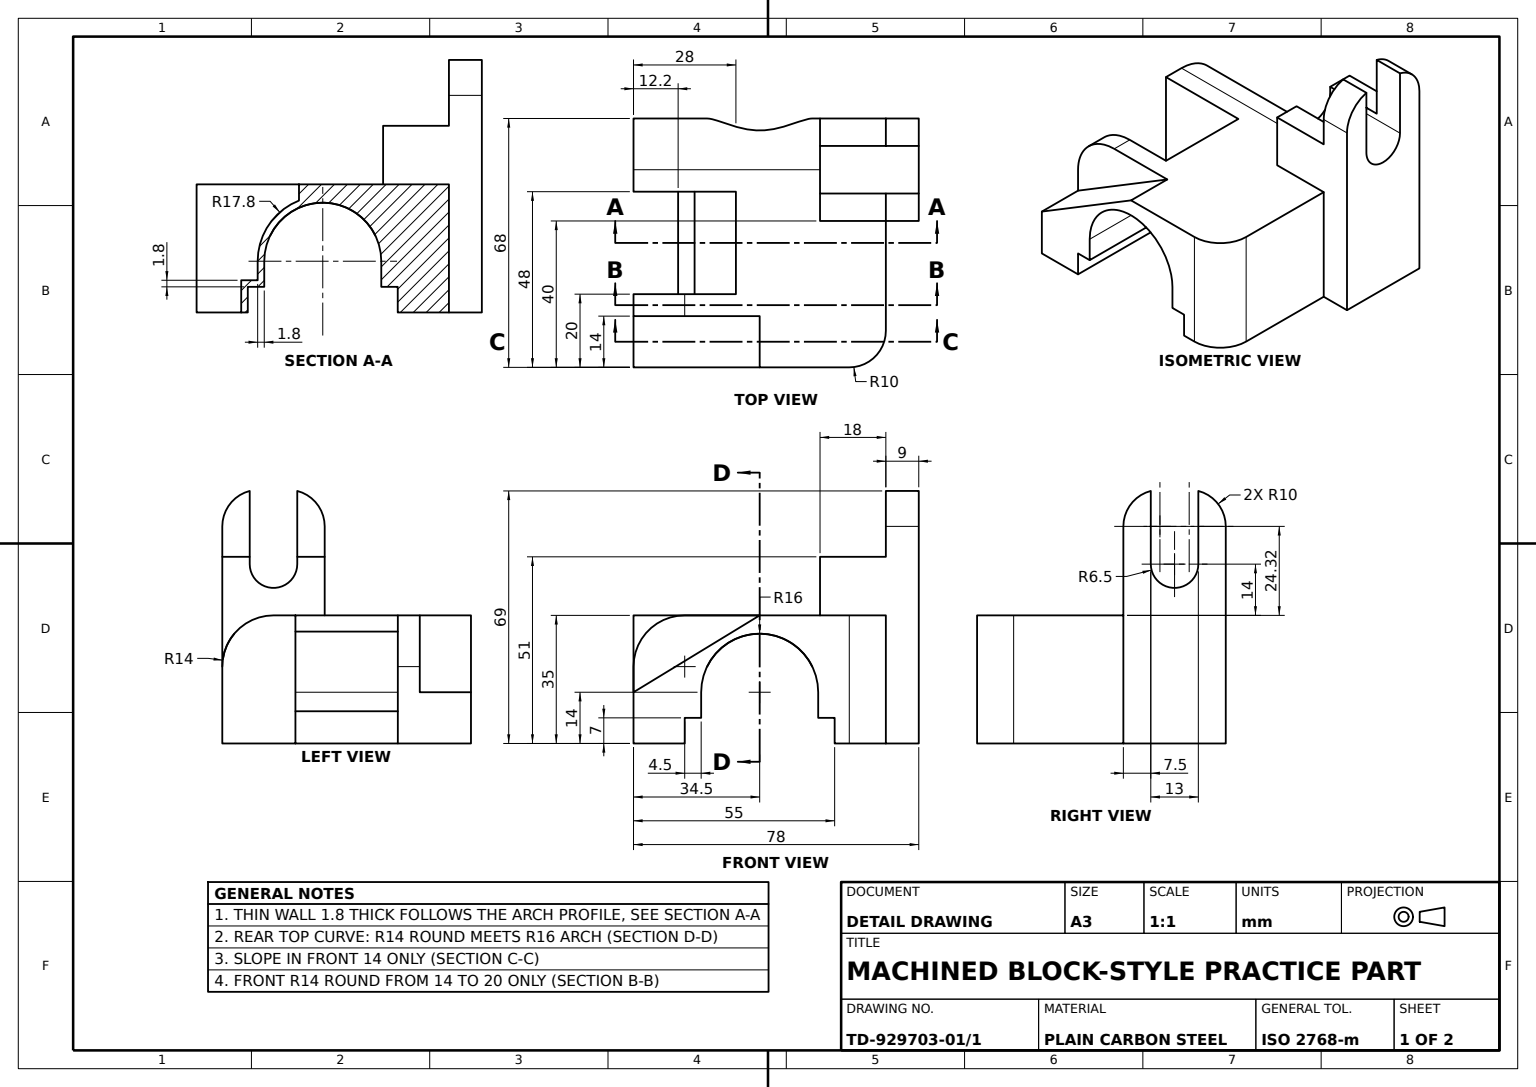
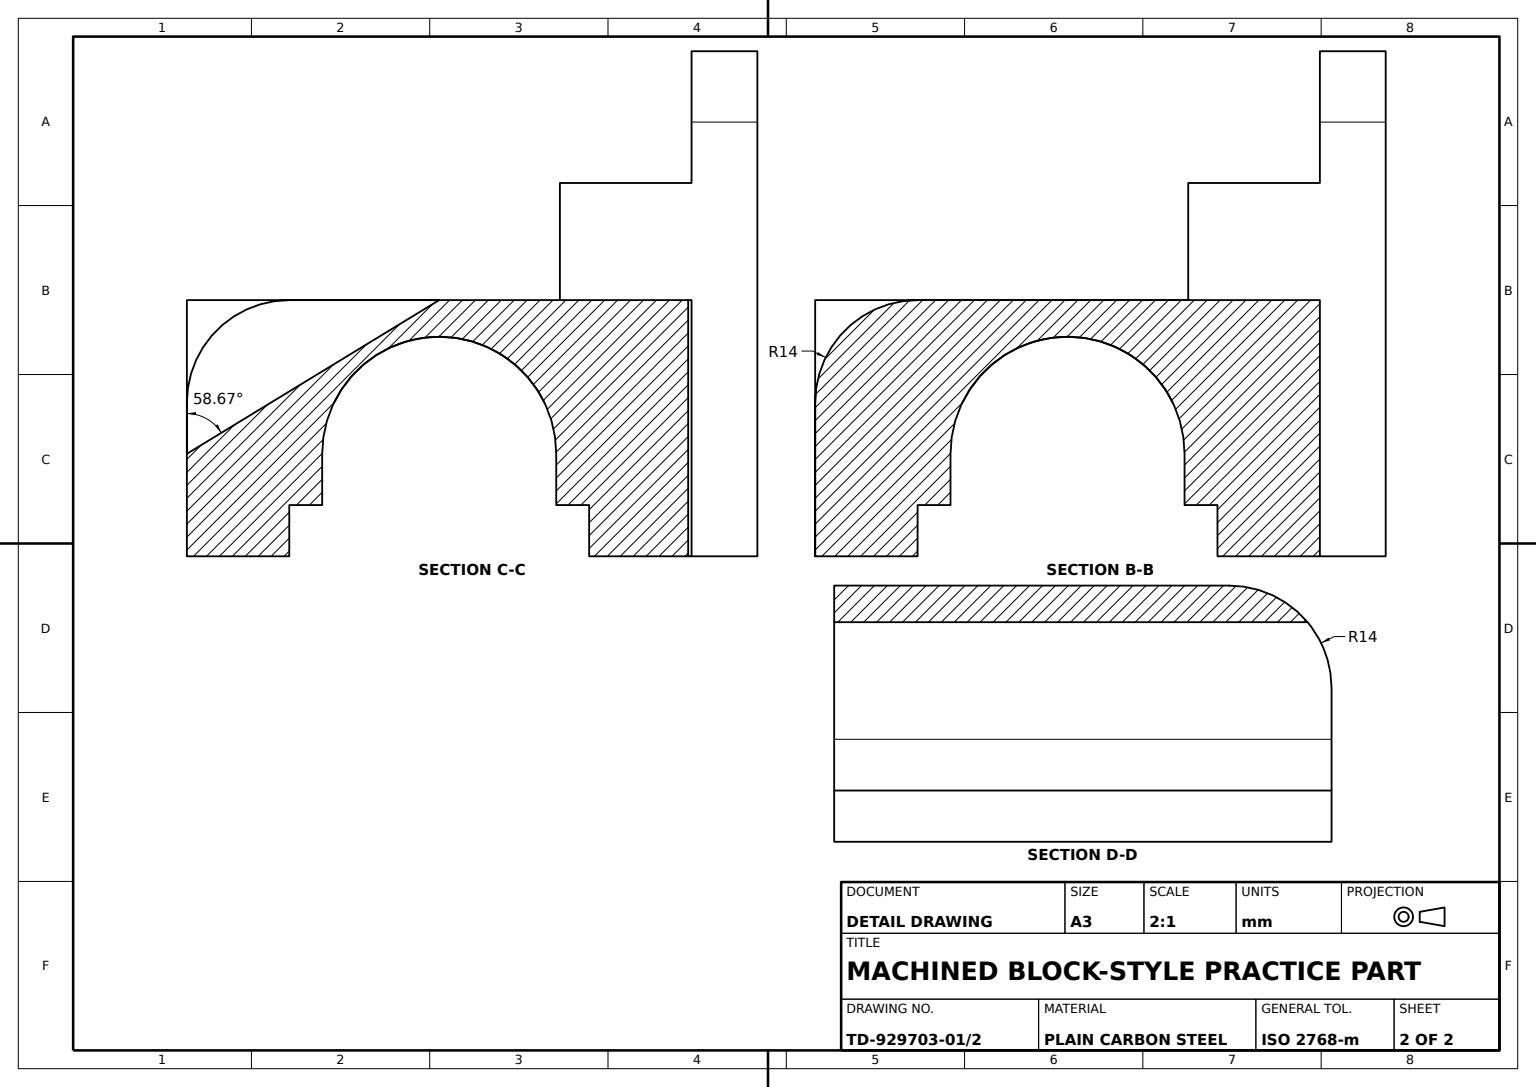
SolidWorks part; units mm, degrees
material "Plain Carbon Steel"
ref_plane "Front Plane" through (0, 0, 0) normal (0, 0, 1) x (1, 0, 0)
ref_plane "Top Plane" through (0, 0, 0) normal (0, 1, 0) x (1, 0, 0)
ref_plane "Right Plane" through (0, 0, 0) normal (1, 0, 0) x (0, 0, -1)
sketch "Base Profile Sketch" plane through (0, 0, 0) normal (1, 0, 0) x (0, 0, -1)
  line L1 (20.5, 0) -> (20.5, 7)
  line L2 (16, 14) -> (16, 7)
  line L3 (16, 7) -> (20.5, 7)
  line L4 (-16, 14) -> (-16, 7)
  line L5 (-16, 7) -> (-20.5, 7)
  line L6 (-20.5, 7) -> (-20.5, 0)
  line L7 (-20.5, 0) -> (-34.5, 0)
  line L8 (-34.5, 0) -> (-34.5, 21)
  line L9 (-20.5, 35) -> (34.5, 35)
  line L10 (34.5, 35) -> (34.5, 0)
  line L11 (34.5, 0) -> (20.5, 0)
  arc A0 (16, 14) -> (-16, 14) centre (0, 14) ccw
  arc A1 (-34.5, 21) -> (-20.5, 35) centre (-20.5, 21) cw
  point P4 (0, 0)
  point P18 (-34.5, 35)
  dimension "D3" = 32
  dimension "D10" = 16
  dimension "D12" = 14
  dimension "D1" = 20.5
  dimension "D2" = 7
  dimension "D4" = 14
  dimension "D5" = 4.5
  dimension "D6" = 7
  dimension "D7" = 69
  dimension "D8" = 35
  dimension "D9" = 34.5
  dimension "D11" = 34.5
extrude "Base Body 20mm" add sketch "Base Profile Sketch" along normal blind 20
sketch "Base Slot Sketch" plane through (20, 0, 0) normal (1, 0, 0) x (0, 0, -1)
  line L1 (34.5, 35) -> (-20.5, 35) construction
  line L3 (-34.5, 21) -> (-34.5, 0) construction
  line L4 (-34.5, 14) -> (0, 35)
  line L5 (-20.5, 35) -> (0, 35)
  line L6 (-34.5, 21) -> (-34.5, 14)
  arc A0 (-34.5, 21) -> (-20.5, 35) centre (-20.5, 21) cw
  dimension "D1" = 14
  dimension "D2" = 7
  dimension "D3" = 40.3887
extrude "Base Slot Cut" cut sketch "Base Slot Sketch" against normal blind 14
sketch "Thin Wall Profile Sketch" plane through (20, 0, 0) normal (1, 0, 0) x (0, 0, -1)
  line L0 (-16, 14) -> (-16, 7)
  line L1 (-16, 7) -> (-20.5, 7)
  line L2 (-20.5, 7) -> (-20.5, 0)
  line L3 (16, 14) -> (16, 7)
  line L4 (16, 7) -> (20.5, 7)
  line L5 (20.5, 7) -> (20.5, 0) construction
  line L6 (16, 7) -> (20.5, 7) construction
  line L7 (20.5, 7) -> (20.5, 0)
  line L20 (-22.3, 8.8) -> (-22.3, 0)
  line L21 (-17.8, 8.8) -> (-22.3, 8.8)
  line L22 (-17.8, 14) -> (-17.8, 8.8)
  line L23 (17.8, 14) -> (17.8, 8.8)
  line L24 (17.8, 8.8) -> (22.3, 8.8)
  line L25 (22.3, 8.8) -> (22.3, 0)
  line L26 (-22.3, 0) -> (-20.5, 0)
  line L27 (20.5, 0) -> (22.3, 0)
  arc A0 (-16, 14) -> (16, 14) centre (0, 14) cw
  arc A2 (-17.8, 14) -> (17.8, 14) centre (0, 14) cw
  dimension "D1" = 1.8
extrude "Thin Wall Boss 1.8mm" add sketch "Thin Wall Profile Sketch" against normal blind 68
sketch "Journal Block Sketch" plane through (0, 0, 34.5) normal (0, 0, 1) x (1, 0, 0)
  line L0 (-48, 0) -> (-28, 0)
  line L1 (-48, 0) -> (0, 0) construction
  line L2 (-28, 0) -> (-28, 35)
  line L3 (-28, 35) -> (-34, 35)
  line L4 (-48, 0) -> (-48, 21)
  line L5 (-48, 31.8) -> (-48, 14) construction
  arc A0 (-48, 21) -> (-34, 35) centre (-34, 21) cw
  dimension "D1" = 14
  dimension "D2" = 35
  dimension "D3" = 20
extrude "Journal Block Boss" add sketch "Journal Block Sketch" against normal blind 69
sketch "Journal Bore Sketch" plane through (20, 0, 0) normal (1, 0, 0) x (0, 0, -1)
  line L0 (-16, 14) -> (-16, 7)
  line L1 (-16, 7) -> (-20.5, 7)
  line L2 (-20.5, 7) -> (-20.5, 0)
  line L3 (-20.5, 0) -> (20.5, 0)
  line L4 (20.5, 0) -> (20.5, 7)
  line L5 (20.5, 7) -> (16, 7)
  line L6 (16, 7) -> (16, 14)
  arc A0 (-16, 14) -> (16, 14) centre (0, 14) cw
extrude "Journal Bore Cut" cut sketch "Journal Bore Sketch" against normal blind 69
sketch "Journal Relief Sketch" plane through (0, 0, 34.5) normal (0, 0, 1) x (1, 0, 0)
  line L0 (-48, 21) -> (-48, 35)
  line L1 (-48, 35) -> (-34, 35)
  arc A0 (-48, 21) -> (-34, 35) centre (-34, 21) cw
extrude "Journal Relief Cut" cut sketch "Journal Relief Sketch" against normal blind 69
sketch "Cross Arm Sketch" plane through (0, 0, -34.5) normal (0, 0, -1) x (-1, 0, 0)
  line L0 (48, 21) -> (48, 35)
  line L1 (48, 35) -> (48, 59)
  line L2 (-20, 35) -> (0, 35) construction
  line L4 (20, 21) -> (20, 59.3175)
  line L5 (27.5, 49) -> (27.5, 69)
  line L7 (40.5, 49) -> (40.5, 69)
  line L9 (48, 59.3175) -> (48, 59)
  line L10 (20, 21) -> (20, 0)
  line L11 (28, 0) -> (0, 0) construction
  line L12 (20, 0) -> (48, 0)
  line L13 (48, 0) -> (48, 21)
  line L15 (28, 35) -> (34, 35) construction
  arc A0 (27.5, 49) -> (40.5, 49) centre (34, 49) ccw
  arc A1 (27.5, 69) -> (20, 59.3175) centre (30, 59.3175) ccw
  arc A2 (40.5, 69) -> (48, 59.3175) centre (38, 59.3175) cw
  point P8 (48, 47)
  dimension "D3" = 13
  dimension "D9" = 10
  dimension "D10" = 10
  dimension "D1" = 24
  dimension "D2" = 14
  dimension "D4" = 14
  dimension "D5" = 14
  dimension "D6" = 24.3175
  dimension "D7" = 14
extrude "Cross Arm Boss" add sketch "Cross Arm Sketch" along normal blind 9
sketch "Upright Lug Sketch" plane through (0, 35, 0) normal (0, 1, 0) x (1, 0, 0)
  line L0 (-28, 34.5) -> (0, 34.5)
  line L3 (0, 34.5) -> (0, -20.5) construction
  line L4 (-28, 34.5) -> (0, 34.5)
  line L5 (-28, 34.5) -> (-28, -6.5)
  line L6 (-28, -6.5) -> (0, -6.5)
  line L7 (0, 34.5) -> (0, -6.5)
  line M3 (-28, -34.5) -> (-28, 34.5)
  dimension "D1" = 41
extrude "Upright Lug Boss" add sketch "Upright Lug Sketch" against normal blind 35 contours L7 L0 L6 M3
sketch "Lug Slot Sketch" plane through (20, 0, 0) normal (1, 0, 0) x (0, 0, -1)
  line L0 (-16, 14) -> (-16, 7)
  line L1 (-16, 7) -> (-20.5, 7)
  line L2 (-20.5, 7) -> (-20.5, 0)
  line L3 (-20.5, 0) -> (20.5, 0)
  line L4 (20.5, 0) -> (20.5, 7)
  line L5 (20.5, 7) -> (16, 7)
  line L6 (16, 7) -> (16, 14)
  arc A0 (-16, 14) -> (16, 14) centre (0, 14) cw
  arc A1 (16, 14) -> (-16, 14) centre (0, 14) ccw construction
extrude "Lug Slot Cut" cut sketch "Lug Slot Sketch" against normal blind 69
sketch "Side Rib Sketch" plane through (0, 0, -34.5) normal (0, 0, 1) x (1, 0, 0)
  line L0 (-20, 35) -> (-20, 51)
  line L1 (-20, 59.3175) -> (-20, 35) construction
  line L2 (-27.5, 49) -> (-27.5, 51)
  line L3 (-27.5, 49) -> (-27.5, 69) construction
  line L4 (-27.5, 51) -> (-20, 51)
  line L5 (-40.5, 49) -> (-40.5, 51)
  line L6 (-40.5, 69) -> (-40.5, 49) construction
  line L7 (-40.5, 51) -> (-48, 51)
  line L8 (-48, 21) -> (-48, 59.3175) construction
  line L9 (-48, 51) -> (-48, 21)
  line L10 (-34, 35) -> (-20, 35)
  arc A0 (-40.5, 49) -> (-27.5, 49) centre (-34, 49) ccw
  arc A1 (-48, 21) -> (-34, 35) centre (-34, 21) cw
  dimension "D1" = 30
  dimension "D3" = 6.5
  dimension "D2" = 16
extrude "Side Rib Boss" add sketch "Side Rib Sketch" along normal blind 18
fillet "Base Edge Fillet R10" radius 10 1 edges at (20, 17.5, -34.5)
